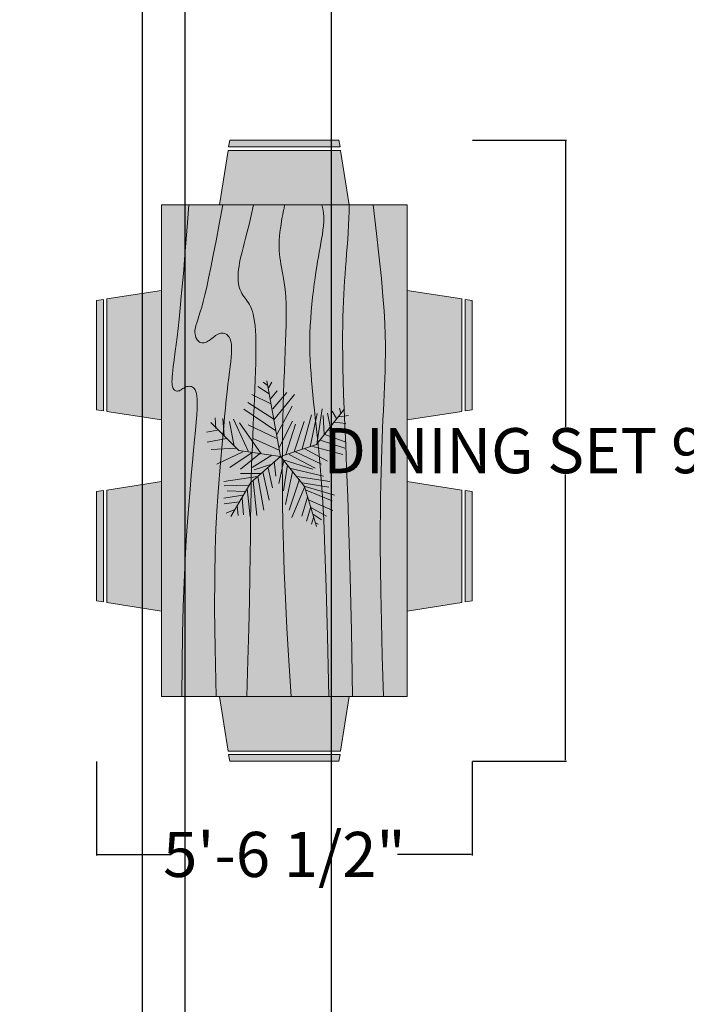
# Model space of a CAD drawing. Units: inches. Extents: x 853 to 1550, y 485 to 1596.
# Tile 9 of 18: x 1170 to 1288, y 1034 to 1208. Entities that reach past the tile are written whole.
import ezdxf

# ---------------------------------------------------------------- set-up
doc = ezdxf.new("R2010")
doc.units = ezdxf.units.IN
doc.header["$MEASUREMENT"] = 0
for name, color, linetype, lineweight in [('A-ANNO-DIMS', 2, 'Continuous', 18), ('furniture', 250, 'Continuous', 18), ('L-PLNT-TREE', 106, 'Continuous', 13)]:
    doc.layers.add(name, color=color, linetype=linetype, lineweight=lineweight)
doc.layers.add('A-FURN-PATT', color=254, linetype='Continuous', lineweight=13, true_color=0xfeeab9)
doc.styles.get("Standard").update_dxf_attribs({"font": 'arial.ttf'})
doc.dimstyles.get("Standard").update_dxf_attribs({"dimtxt": 8, "dimasz": 0.18, "dimexe": 0.18, "dimexo": 0.0625, "dimgap": 0.09, "dimtad": 0, "dimtih": 1, "dimtoh": 1, "dimzin": 0, "dimdsep": 46, "dimlunit": 3, "dimtxsty": 'Standard', "dimcen": 0.09, "dimadec": 0, "dimazin": 0, "dimtfac": 1, "dimtofl": 0, "dimtmove": 0, "dimatfit": 3, "dimfxl": 1, "dimtolj": 1, "dimtzin": 0, "dimarcsym": 0})

# ---------------------------------------------------------------- blocks, each defined once
blk = doc.blocks.new('Dining Set - 36 x 72 in.')
for p, q in [((-22, 27.5), (-22.1562, 26.50042)), ((-22, 27.5), (-6, 27.5)), ((-5.8437, 26.49966), (-6, 27.5)), ((6, 27.5), (5.8438, 26.50042)), ((6, 27.5), (22, 27.5)), ((22.1563, 26.49966), (22, 27.5)), ((-22.2343, 26.00059), (-23.4847, 17.99762)), ((-22.2304, 26), (-5.7608, 26)), ((-5.8416, 26.5), (-22.1534, 26.5)), ((-4.5152, 17.99762), (-5.7655, 25.99926)), ((5.7657, 26.00059), (4.5153, 17.99762)), ((5.7696, 26), (22.2392, 26)), ((22.1584, 26.5), (5.8466, 26.5)), ((23.4848, 17.99762), (22.2345, 25.99926)), ((36, 18), (-36, 18)), ((-36, 18), (-36, -18)), ((36, -18), (36, 18)), ((-44.0006, 8.23428), (-35.9976, 9.48474)), ((44.0006, 8.23428), (35.9976, 9.48474)), ((-45.5, 8), (-44.5004, 8.15617)), ((-45.5, 8), (-45.5, -8)), ((-44.5, -8.15843), (-44.5, 8.15338)), ((-44, 8.23041), (-44, -8.23915)), ((44, 8.23041), (44, -8.23915)), ((44.5, -8.15843), (44.5, 8.15338)), ((45.5, 8), (44.5005, 8.15617)), ((45.5, 8), (45.5, -8)), ((-44.4997, -8.15631), (-45.5, -8)), ((-35.9976, -9.48476), (-43.9993, -8.2345)), ((35.9976, -9.48476), (43.9993, -8.2345)), ((44.4997, -8.15631), (45.5, -8)), ((-36, -18), (36, -18)), ((-22.2343, -26.0006), (-23.4847, -17.99762)), ((-4.5152, -17.99762), (-5.7655, -25.99928)), ((5.7657, -26.0006), (4.5153, -17.99762)), ((23.4848, -17.99762), (22.2345, -25.99928)), ((-22.2304, -26), (-5.7608, -26)), ((-22, -27.5), (-22.1562, -26.50044)), ((-5.8416, -26.5), (-22.1534, -26.5)), ((-5.8437, -26.49967), (-6, -27.5)), ((5.7696, -26), (22.2392, -26)), ((6, -27.5), (5.8438, -26.50044)), ((22.1584, -26.5), (5.8466, -26.5)), ((22.1563, -26.49967), (22, -27.5)), ((-22, -27.5), (-6, -27.5)), ((6, -27.5), (22, -27.5))]:
    blk.add_line(p, q)
for points in [[(-36, 15), (-31.1772, 14.97754), (-26.8079, 14.91406), (-22.8538, 14.81543), (-19.276, 14.6875), (-16.0362, 14.53613), (-13.0957, 14.36718), (-10.4159, 14.18652), (-7.9583, 14), (-5.6904, 13.81315), (-3.6035, 13.63021), (-1.6954, 13.45508), (0.0365, 13.29166), (1.5945, 13.14388), (2.9811, 13.01562), (4.1988, 12.9108), (5.25, 12.83333), (6.1393, 12.78613), (6.8802, 12.76823), (7.4883, 12.77767), (7.9792, 12.8125), (8.3685, 12.87077), (8.6719, 12.95052), (8.9049, 13.0498), (9.0833, 13.16666), (9.2205, 13.29899), (9.3216, 13.44401), (9.3895, 13.59879), (9.4271, 13.76041), (9.4373, 13.92594), (9.4232, 14.09245), (9.3875, 14.257), (9.3333, 14.41666), (9.2638, 14.56917), (9.1836, 14.71484), (9.0975, 14.85465), (9.0104, 14.98958), (8.9272, 15.1206), (8.8529, 15.2487), (8.7922, 15.37483), (8.75, 15.5), (8.7305, 15.62467), (8.7344, 15.74739), (8.7617, 15.86621), (8.8125, 15.97916), (8.8867, 16.08431), (8.9844, 16.17968), (9.1055, 16.26334), (9.25, 16.33333), (9.4189, 16.38802), (9.6172, 16.42708), (9.8506, 16.45052), (10.125, 16.45833), (10.4463, 16.45052), (10.8203, 16.42708), (11.2529, 16.38802), (11.75, 16.33333), (12.3184, 16.26318), (12.9694, 16.17838), (13.7151, 16.07991), (14.5677, 15.96875), (15.5395, 15.84586), (16.6426, 15.71224), (17.8893, 15.56884), (19.2917, 15.41666), (20.859, 15.25667), (22.5879, 15.08984), (24.4721, 14.91715), (26.5052, 14.73958), (28.6809, 14.5581), (30.9929, 14.3737), (33.4347, 14.18733), (36, 14)], [(-36, 10), (-28.9766, 10.14274), (-23.1725, 10.20442), (-18.4241, 10.19775), (-14.5677, 10.13541), (-11.4399, 10.03011), (-8.877, 9.89453), (-6.7154, 9.74137), (-4.7917, 9.58333), (-2.9698, 9.43082), (-1.2246, 9.28515), (0.4415, 9.14534), (2.026, 9.01041), (3.5266, 8.87939), (4.9408, 8.7513), (6.266, 8.62516), (7.5, 8.5), (8.6411, 8.37549), (9.6914, 8.2539), (10.6538, 8.13818), (11.5312, 8.03125), (12.3267, 7.93603), (13.043, 7.85547), (13.6831, 7.79248), (14.25, 7.75), (14.7471, 7.7303), (15.1797, 7.73307), (15.5537, 7.75732), (15.875, 7.80208), (16.1494, 7.86637), (16.3828, 7.94922), (16.5811, 8.04964), (16.75, 8.16666), (16.8944, 8.29915), (17.0143, 8.44531), (17.1089, 8.60319), (17.1771, 8.77083), (17.218, 8.94629), (17.2305, 9.1276), (17.2137, 9.31282), (17.1667, 9.5), (17.0895, 9.6875), (16.987, 9.875), (16.8649, 10.0625), (16.7292, 10.25), (16.5856, 10.4375), (16.4401, 10.625), (16.2985, 10.8125), (16.1667, 11), (16.05, 11.18733), (15.9518, 11.3737), (15.8752, 11.5581), (15.8229, 11.73958), (15.798, 11.91715), (15.8034, 12.08984), (15.842, 12.25667), (15.9167, 12.41666), (16.0295, 12.56836), (16.1784, 12.70833), (16.3605, 12.83268), (16.5729, 12.9375), (16.8127, 13.01888), (17.0768, 13.07291), (17.3625, 13.0957), (17.6667, 13.08333), (17.9894, 13.03312), (18.3418, 12.94726), (18.7382, 12.82918), (19.1927, 12.68229), (19.7195, 12.51001), (20.3327, 12.31575), (21.0465, 12.10294), (21.875, 11.875), (22.8357, 11.63354), (23.959, 11.37304), (25.2786, 11.08618), (26.8282, 10.76562), (28.6414, 10.40405), (30.752, 9.99414), (33.1936, 9.52856), (36, 9)], [(-36, 5.5), (-30.7157, 5.3348), (-26.069, 5.20963), (-21.9946, 5.11767), (-18.4271, 5.05208), (-15.3009, 5.00602), (-12.5508, 4.97265), (-10.1112, 4.94515), (-7.9167, 4.91666), (-5.909, 4.88167), (-4.0586, 4.83984), (-2.3429, 4.79215), (-0.7396, 4.73958), (0.7739, 4.6831), (2.22, 4.6237), (3.6213, 4.56233), (5, 4.5), (6.373, 4.43782), (7.7344, 4.3776), (9.0723, 4.32129), (10.375, 4.27083), (11.6309, 4.22819), (12.8281, 4.19531), (13.9551, 4.17415), (15, 4.16666), (15.954, 4.17448), (16.819, 4.19791), (17.6001, 4.23698), (18.3021, 4.29166), (18.9299, 4.36198), (19.4883, 4.44791), (19.9823, 4.54948), (20.4167, 4.66666), (20.7969, 4.79899), (21.1302, 4.94401), (21.4245, 5.09879), (21.6875, 5.26041), (21.9271, 5.42594), (22.1511, 5.59245), (22.3672, 5.757), (22.5834, 5.91666), (22.8065, 6.06868), (23.0404, 6.21093), (23.2879, 6.34147), (23.5521, 6.45833), (23.8358, 6.55957), (24.142, 6.64323), (24.4735, 6.70735), (24.8334, 6.75), (25.2235, 6.76969), (25.642, 6.76692), (26.0858, 6.74267), (26.5521, 6.69791), (27.0379, 6.63362), (27.5404, 6.55078), (28.0565, 6.45036), (28.5834, 6.33333), (29.1242, 6.19987), (29.7071, 6.04687), (30.3661, 5.87044), (31.1354, 5.66666), (32.0493, 5.43164), (33.142, 5.16146), (34.4475, 4.85221), (36, 4.5)], [(-36, -1), (-30.7915, -0.6591), (-26.0195, -0.38216), (-21.6519, -0.16284), (-17.6563, 0.00521), (-14.0005, 0.12833), (-10.6523, 0.21289), (-7.5796, 0.26522), (-4.75, 0.29166), (-2.134, 0.29793), (0.2878, 0.28711), (2.5317, 0.26163), (4.6146, 0.22396), (6.5529, 0.17651), (8.3633, 0.12174), (10.0623, 0.06209), (11.6667, 0), (13.1899, -0.06201), (14.6341, -0.1211), (15.9982, -0.17432), (17.2813, -0.21875), (18.4823, -0.25147), (19.6003, -0.26953), (20.6343, -0.27002), (21.5834, -0.25), (22.4481, -0.20768), (23.2357, -0.14584), (23.9549, -0.06836), (24.6146, 0.02083), (25.2235, 0.11784), (25.7904, 0.21875), (26.3241, 0.31966), (26.8334, 0.41666), (27.3265, 0.50618), (27.8099, 0.58593), (28.2894, 0.65397), (28.7709, 0.70833), (29.2601, 0.74707), (29.763, 0.76823), (30.2855, 0.76985), (30.8334, 0.75), (31.4088, 0.70784), (31.9994, 0.64713), (32.589, 0.57275), (33.1615, 0.48958), (33.7008, 0.4025), (34.1908, 0.3164), (34.6153, 0.23616), (34.9584, 0.16666), (35.2099, 0.11165), (35.3848, 0.07031), (35.504, 0.04069), (35.5886, 0.02083), (35.6594, 0.00879), (35.7377, 0.0026), (35.8442, 0.00032), (36, 0)], [(-36, -6.5), (-27.1843, -6.31267), (-20.084, -6.1263), (-14.469, -5.9419), (-10.1094, -5.76042), (-6.7752, -5.58285), (-4.2363, -5.41016), (-2.2629, -5.24333), (-0.625, -5.08334), (0.8708, -4.93099), (2.2715, -4.78646), (3.5872, -4.64974), (4.8281, -4.52084), (6.0046, -4.39974), (7.127, -4.28646), (8.2053, -4.18099), (9.25, -4.08334), (10.2705, -3.99382), (11.2734, -3.91407), (12.2647, -3.84603), (13.25, -3.79167), (14.2354, -3.75293), (15.2266, -3.73177), (16.2295, -3.73015), (17.25, -3.75), (18.2912, -3.79248), (19.3451, -3.85547), (20.4009, -3.93604), (21.4479, -4.03125), (22.4754, -4.13819), (23.4727, -4.25391), (24.4289, -4.37549), (25.3334, -4.5), (26.1785, -4.62492), (26.9694, -4.74935), (27.7145, -4.87281), (28.4219, -4.99479), (29.1, -5.11483), (29.7572, -5.23242), (30.4016, -5.34709), (31.0417, -5.45834), (31.6837, -5.56437), (32.3262, -5.65821), (32.9658, -5.73153), (33.599, -5.77604), (34.2224, -5.78345), (34.8327, -5.74545), (35.4264, -5.65373), (36, -5.5)], [(-36, -10), (-26.4022, -9.81299), (-18.4675, -9.62891), (-11.9839, -9.45069), (-6.7396, -9.28125), (-2.5226, -9.12354), (0.8789, -8.98047), (3.6769, -8.85498), (6.0833, -8.75), (8.2767, -8.66765), (10.3021, -8.60677), (12.1712, -8.56543), (13.8958, -8.54167), (15.4876, -8.53353), (16.9583, -8.53907), (18.3197, -8.55632), (19.5834, -8.58334), (20.7616, -8.61841), (21.8685, -8.66081), (22.9188, -8.71004), (23.9271, -8.76563), (24.9081, -8.82707), (25.8763, -8.89388), (26.8465, -8.96558), (27.8334, -9.04167), (28.8474, -9.12118), (29.8828, -9.20117), (30.93, -9.27824), (31.9792, -9.34896), (33.0205, -9.40991), (34.0443, -9.45768), (35.0407, -9.48885), (36, -9.5)], [(-36, -14.5), (-30.0881, -14.33513), (-25.0332, -14.21224), (-20.7312, -14.12647), (-17.0781, -14.07292), (-13.97, -14.04671), (-11.3027, -14.04297), (-8.9724, -14.05681), (-6.875, -14.08334), (-4.9224, -14.11833), (-3.0905, -14.16016), (-1.3709, -14.20785), (0.2448, -14.26042), (1.7647, -14.3169), (3.1973, -14.3763), (4.5507, -14.43767), (5.8333, -14.5), (7.0554, -14.5621), (8.235, -14.62175), (9.3922, -14.67652), (10.5469, -14.72396), (11.7192, -14.76164), (12.929, -14.78711), (14.1965, -14.79794), (15.5417, -14.79167), (16.9933, -14.76424), (18.6152, -14.70508), (20.4804, -14.60197), (22.6615, -14.44271), (25.2312, -14.21509), (28.2624, -13.9069), (31.8277, -13.50594), (36, -13)]]:
    blk.add_lwpolyline(points)
blk = doc.blocks.new('dining area')
at = {"layer": 'furniture', "xscale": 0.6659924291999282, "yscale": 0.6659924291999282, "zscale": 0.6659924291999282, "rotation": 90}
blk.add_blockref('Dining Set - 36 x 72 in.', (-0.439, 20.507), dxfattribs=at)
blk = doc.blocks.new('*U18')
for p, q in [((-8.737, 47.138), (-17.069, 52.711)), ((-10.186, 53.64), (-13.084, 55.962)), ((0, 0), (-10.5, 57)), ((-9.099, 51.782), (-6.563, 55.962)), ((-7.288, 39.707), (-21.778, 46.673)), ((-7.65, 43.423), (-2.578, 49.46)), ((-5.839, 35.992), (4.667, 48.067)), ((-5.114, 27.632), (10.463, 46.673)), ((-5.114, 28.097), (-24.676, 40.636)), ((-2.941, 16.486), (8.652, 37.85)), ((-3.665, 19.273), (-27.574, 35.527)), ((16.259, 5.805), (23.142, 31.348)), ((22.055, 7.198), (27.489, 32.277)), ((27, 9), (48, 36)), ((27.127, 9.056), (31.112, 35.992)), ((31.836, 30.883), (32.561, 16.486)), ((35.096, 32.741), (37.27, 22.524)), ((38.719, 34.134), (41.979, 28.561)), ((43.791, 29.954), (51.036, 30.883)), ((44.153, 36.456), (45.239, 32.741)), ((-31.5, 4.5), (-52.5, 25.5)), ((-48.585, 21.131), (-49.309, 29.026)), ((-43.513, 28.561), (-42.427, 15.558)), ((-38.442, 26.239), (-34.819, 7.663)), ((-35.544, 28.097), (-24.314, 3.947)), ((-14.533, 2.09), (-30.834, 25.31)), ((-24.314, 23.917), (-2.941, 13.7)), ((-1.129, 6.734), (9.014, 26.704)), ((3.942, 1.625), (11.187, 24.381)), ((10.101, 3.483), (17.708, 26.239)), ((40.53, 25.775), (48.862, 24.846)), ((-47.498, 19.737), (-55.83, 18.344)), ((33.285, 16.486), (48.862, 10.913)), ((36.183, 19.737), (48.137, 17.88)), ((-40.615, 13.7), (-55.105, 10.913)), ((-20.691, 13.7), (-1.129, 4.876)), ((0, 0), (27, 9)), ((24.229, 7.663), (46.688, 1.625)), ((29.662, 12.307), (48.137, 6.269)), ((-33.37, 6.269), (-52.207, 5.34)), ((-28.299, 3.483), (-47.86, -5.805)), ((-21.416, 3.018), (-38.079, -8.128)), ((0, 0), (-31.5, 4.5)), ((-15.982, 2.09), (-30.11, -9.521)), ((0, 0), (-22.5, -19.5)), ((-6.563, 1.161), (-21.416, -8.128)), ((0, 0), (18, -22.5)), ((6.478, 1.625), (26.04, -8.592)), ((11.187, 3.483), (30.749, -5.805)), ((18.07, 5.805), (35.096, -3.483)), ((-6.563, -5.805), (-19.967, -9.985)), ((-4.752, -3.483), (-3.665, -14.629)), ((2.493, -3.019), (-1.491, -20.202)), ((1.769, -2.555), (24.229, -9.521)), ((5.029, -6.27), (2.131, -25.775)), ((-15.257, -12.772), (-30.11, -12.772)), ((-13.446, -11.378), (-8.737, -32.741)), ((-9.461, -8.592), (-6.201, -23.453)), ((9.014, -11.378), (3.58, -35.992)), ((7.565, -9.056), (32.198, -14.629)), ((-17.431, -15.094), (-42.789, -18.809)), ((-24.314, -21.596), (-42.427, -22.06)), ((-22.5, -19.5), (-37.5, -45)), ((-20.691, -18.345), (-17.793, -44.352)), ((-17.069, -15.094), (-12.721, -40.172)), ((14.085, -16.951), (6.478, -40.172)), ((12.274, -15.094), (36.907, -18.809)), ((16.259, -19.738), (36.183, -22.989)), ((-28.299, -29.026), (-42.789, -31.348)), ((-26.849, -26.24), (-40.253, -25.775)), ((-25.038, -23.918), (-22.865, -45.281)), ((18.07, -22.524), (8.289, -45.745)), ((18, -22.5), (27, -52.5)), ((18.433, -22.524), (40.53, -29.026)), ((19.157, -25.311), (38.719, -33.206)), ((-30.834, -34.135), (-42.427, -35.528)), ((-32.646, -36.921), (-31.921, -44.352)), ((-29.023, -30.884), (-27.936, -43.887)), ((20.244, -30.419), (15.897, -44.816)), ((21.331, -32.741), (39.081, -40.636)), ((-34.457, -39.708), (-40.978, -42.494)), ((22.78, -37.85), (19.519, -48.532)), ((22.78, -38.314), (34.372, -44.816)), ((24.591, -43.423), (30.749, -47.603)), ((24.591, -45.745), (23.142, -50.854)), ((26.764, -49.925), (28.213, -50.854))]:
    blk.add_line(p, q)
blk = doc.blocks.new('*D67')
at = {"layer": 'A-ANNO-DIMS', "color": 0, "lineweight": -2, "transparency": 16777216}
for p, q in [((1250.4, 1186.71), (1267.03, 1186.71)), ((1266.85, 1186.53), (1266.85, 1135.89)), ((1266.85, 1076.81), (1266.85, 1127.44)), ((1250.4, 1076.63), (1267.03, 1076.63))]:
    blk.add_line(p, q, dxfattribs=at)
at = {"layer": 'A-ANNO-DIMS', "color": 0, "transparency": 16777216}
for points in [[(1266.82, 1186.53), (1266.88, 1186.53), (1266.85, 1186.71)], [(1266.82, 1076.81), (1266.88, 1076.81), (1266.85, 1076.63)]]:
    blk.add_solid(points, dxfattribs=at)
at = {"layer": 'Defpoints', "color": 0, "transparency": 16777216}
for p in [(1250.34, 1186.71), (1266.85, 1186.71), (1250.34, 1076.63)]:
    blk.add_point(p, dxfattribs=at)
at = {"layer": 'A-ANNO-DIMS', "color": 0, "transparency": 16777216, "insert": (1266.85, 1131.67), "char_height": 8, "attachment_point": 5}
blk.add_mtext('\\A1;DINING SET 9\'-2"', dxfattribs=at)
blk = doc.blocks.new('*D68')
at = {"layer": 'A-ANNO-DIMS', "color": 0, "lineweight": -2, "transparency": 16777216}
for p, q in [((1183.81, 1076.57), (1183.81, 1059.94)), ((1250.34, 1076.57), (1250.34, 1059.94)), ((1183.99, 1060.12), (1197.03, 1060.12)), ((1250.16, 1060.12), (1237.12, 1060.12))]:
    blk.add_line(p, q, dxfattribs=at)
at = {"layer": 'A-ANNO-DIMS', "color": 0, "transparency": 16777216}
for points in [[(1183.99, 1060.15), (1183.99, 1060.09), (1183.81, 1060.12)], [(1250.16, 1060.15), (1250.16, 1060.09), (1250.34, 1060.12)]]:
    blk.add_solid(points, dxfattribs=at)
at = {"layer": 'Defpoints', "color": 0, "transparency": 16777216}
for p in [(1183.81, 1076.63), (1250.34, 1076.63), (1250.34, 1060.12)]:
    blk.add_point(p, dxfattribs=at)
at = {"layer": 'A-ANNO-DIMS', "color": 0, "transparency": 16777216, "insert": (1217.08, 1060.12), "char_height": 8, "attachment_point": 5}
blk.add_mtext('\\A1;5\'-6 1/2"', dxfattribs=at)
blk = doc.blocks.new('*D72')
at = {"layer": 'A-ANNO-DIMS', "color": 0, "lineweight": -2, "transparency": 16777216}
for p, q in [((1139.44, 1321.07), (1139.44, 497.1)), ((1199.44, 1321.07), (1199.44, 497.1)), ((1139.62, 497.28), (1158.71, 497.28)), ((1199.26, 497.28), (1180.16, 497.28))]:
    blk.add_line(p, q, dxfattribs=at)
at = {"layer": 'A-ANNO-DIMS', "color": 0, "transparency": 16777216}
for points in [[(1139.62, 497.31), (1139.62, 497.25), (1139.44, 497.28)], [(1199.26, 497.31), (1199.26, 497.25), (1199.44, 497.28)]]:
    blk.add_solid(points, dxfattribs=at)
at = {"layer": 'Defpoints', "color": 0, "transparency": 16777216}
for p in [(1139.44, 1321.13), (1199.44, 1321.13), (1199.44, 497.28)]:
    blk.add_point(p, dxfattribs=at)
at = {"layer": 'A-ANNO-DIMS', "color": 0, "transparency": 16777216, "insert": (1169.44, 497.28), "char_height": 8, "attachment_point": 5}
blk.add_mtext('\\A1;5\'-0"', dxfattribs=at)
blk = doc.blocks.new('*D81')
at = {"layer": 'A-ANNO-DIMS', "color": 0, "lineweight": -2, "transparency": 16777216}
for p, q in [((1191.94, 767.69), (1191.94, 1584.65)), ((1192.12, 1584.47), (1225.27, 1584.47)), ((1225.45, 767.69), (1225.45, 1584.65)), ((1225.45, 1584.47), (1225.63, 1584.47))]:
    blk.add_line(p, q, dxfattribs=at)
at = {"layer": 'A-ANNO-DIMS', "color": 0, "transparency": 16777216}
for points in [[(1192.12, 1584.5), (1192.12, 1584.44), (1191.94, 1584.47)], [(1225.27, 1584.5), (1225.27, 1584.44), (1225.45, 1584.47)]]:
    blk.add_solid(points, dxfattribs=at)
at = {"layer": 'Defpoints', "color": 0, "transparency": 16777216}
for p in [(1225.45, 1584.47), (1191.94, 767.63), (1225.45, 767.63)]:
    blk.add_point(p, dxfattribs=at)
at = {"layer": 'A-ANNO-DIMS', "color": 0, "transparency": 16777216, "insert": (1245.74, 1584.47), "char_height": 8, "attachment_point": 5}
blk.add_mtext('\\A1;2\'-9 1/2"', dxfattribs=at)

msp = doc.modelspace()

# ---------------------------------------------------------------- hatches: boundary and pattern name
at = {"layer": 'A-FURN-PATT'}
h = msp.add_hatch(color=256, dxfattribs=at)
h.dxf.hatch_style = 1
h.paths.add_polyline_path([(1195.302, 1126.206), (1185.625, 1124.693), (1185.625, 1104.772), (1195.302, 1103.26)])
h.paths.add_polyline_path([(1195.302, 1160.075), (1185.625, 1158.563), (1185.625, 1138.642), (1195.302, 1137.13)])
h.paths.add_polyline_path([(1248.526, 1158.563), (1238.849, 1160.075), (1238.849, 1137.13), (1248.526, 1138.642)])
h.paths.add_polyline_path([(1248.526, 1124.693), (1238.849, 1126.206), (1238.849, 1103.26), (1248.526, 1104.772)])
h.paths.add_polyline_path([(1228.548, 1088.121), (1205.602, 1088.121), (1207.114, 1078.444), (1227.036, 1078.444)])
h.paths.add_polyline_path([(1227.036, 1184.892), (1207.114, 1184.892), (1205.602, 1175.215), (1228.548, 1175.215)])
h.paths.add_polyline_path([(1226.752, 1186.706), (1207.398, 1186.706), (1207.209, 1185.496), (1226.941, 1185.496)])
h.paths.add_polyline_path([(1185.02, 1158.469), (1183.81, 1158.28), (1183.81, 1138.926), (1185.02, 1138.736)])
h.paths.add_polyline_path([(1185.02, 1124.599), (1183.81, 1124.41), (1183.81, 1105.056), (1185.02, 1104.867)])
h.paths.add_polyline_path([(1226.941, 1077.839), (1207.209, 1077.839), (1207.398, 1076.629), (1226.752, 1076.629)])
h.paths.add_polyline_path([(1250.34, 1124.41), (1249.13, 1124.599), (1249.13, 1104.867), (1250.34, 1105.056)])
h.paths.add_polyline_path([(1250.34, 1158.28), (1249.13, 1158.469), (1249.13, 1138.736), (1250.34, 1138.926)])
h = msp.add_hatch(color=256, dxfattribs=at)
h.dxf.hatch_style = 1
h.paths.add_polyline_path([(1200.997, 1131.712), (1201.176, 1133.596), (1201.331, 1135.274), (1201.458, 1136.747), (1201.551, 1138.018), (1201.609, 1139.094), (1201.63, 1139.99), (1201.619, 1140.726), (1201.577, 1141.32), (1201.506, 1141.791), (1201.41, 1142.158), (1201.29, 1142.439), (1201.148, 1142.655), (1200.988, 1142.821), (1200.813, 1142.943), (1200.626, 1143.026), (1200.43, 1143.071), (1200.23, 1143.083), (1200.028, 1143.066), (1199.829, 1143.023), (1199.636, 1142.958), (1199.452, 1142.874), (1199.275, 1142.777), (1199.106, 1142.672), (1198.81, 1142.481), (1198.539, 1142.324), (1198.249, 1142.226), (1197.951, 1142.236), (1197.676, 1142.359), (1197.444, 1142.597), (1197.318, 1142.857), (1197.252, 1143.061), (1197.204, 1143.301), (1197.176, 1143.583), (1197.167, 1143.915), (1197.176, 1144.304), (1197.204, 1144.756), (1197.252, 1145.28), (1197.318, 1145.881), (1197.403, 1146.568), (1197.505, 1147.356), (1197.624, 1148.258), (1197.759, 1149.289), (1197.907, 1150.465), (1198.069, 1151.799), (1198.242, 1153.307), (1198.427, 1155.004), (1198.62, 1156.899), (1198.822, 1158.991), (1199.031, 1161.27), (1199.246, 1163.729), (1199.465, 1166.361), (1199.688, 1169.158), (1199.914, 1172.111), (1200.14, 1175.215), (1195.302, 1175.215), (1195.302, 1088.121), (1198.931, 1088.121), (1198.958, 1093.955), (1199.035, 1099.24), (1199.154, 1104.023), (1199.309, 1108.351), (1199.492, 1112.27), (1199.696, 1115.827), (1199.915, 1119.068), (1200.14, 1122.041), (1200.366, 1124.784), (1200.588, 1127.309), (1200.799, 1129.617)])
h.paths.add_polyline_path([(1207.091, 1143.391), (1207.231, 1144.555), (1207.36, 1145.616), (1207.475, 1146.579), (1207.573, 1147.445), (1207.649, 1148.219), (1207.7, 1148.905), (1207.724, 1149.506), (1207.721, 1150.03), (1207.692, 1150.482), (1207.637, 1150.871), (1207.56, 1151.203), (1207.459, 1151.485), (1207.338, 1151.725), (1207.196, 1151.929), (1207.036, 1152.104), (1206.859, 1152.249), (1206.668, 1152.363), (1206.466, 1152.446), (1206.253, 1152.495), (1206.034, 1152.51), (1205.81, 1152.49), (1205.584, 1152.433), (1205.357, 1152.34), (1205.13, 1152.216), (1204.903, 1152.068), (1204.676, 1151.904), (1204.45, 1151.73), (1204.223, 1151.554), (1203.996, 1151.383), (1203.769, 1151.224), (1203.542, 1151.082), (1203.317, 1150.964), (1203.094, 1150.871), (1202.874, 1150.808), (1202.547, 1150.762), (1202.249, 1150.831), (1202.055, 1150.921), (1201.872, 1151.058), (1201.703, 1151.238), (1201.552, 1151.458), (1201.425, 1151.715), (1201.327, 1152.005), (1201.262, 1152.324), (1201.234, 1152.67), (1201.249, 1153.038), (1201.31, 1153.428), (1201.414, 1153.855), (1201.556, 1154.334), (1201.734, 1154.884), (1201.943, 1155.521), (1202.178, 1156.263), (1202.435, 1157.126), (1202.711, 1158.128), (1203.003, 1159.291), (1203.318, 1160.649), (1203.665, 1162.246), (1204.053, 1164.12), (1204.49, 1166.313), (1204.986, 1168.866), (1205.549, 1171.82), (1206.188, 1175.215), (1200.14, 1175.215), (1199.914, 1172.111), (1199.688, 1169.158), (1199.465, 1166.361), (1199.246, 1163.729), (1199.031, 1161.27), (1198.822, 1158.991), (1198.62, 1156.899), (1198.427, 1155.004), (1198.242, 1153.307), (1198.069, 1151.799), (1197.907, 1150.465), (1197.759, 1149.289), (1197.624, 1148.258), (1197.505, 1147.356), (1197.403, 1146.568), (1197.318, 1145.881), (1197.252, 1145.28), (1197.204, 1144.756), (1197.176, 1144.304), (1197.167, 1143.915), (1197.176, 1143.583), (1197.204, 1143.301), (1197.252, 1143.061), (1197.318, 1142.857), (1197.402, 1142.682), (1197.504, 1142.536), (1197.619, 1142.417), (1197.746, 1142.328), (1197.883, 1142.266), (1198.026, 1142.233), (1198.175, 1142.228), (1198.326, 1142.252), (1198.477, 1142.303), (1198.63, 1142.376), (1198.785, 1142.466), (1198.943, 1142.567), (1199.223, 1142.747), (1199.553, 1142.929), (1199.933, 1143.058), (1200.338, 1143.093), (1200.626, 1143.026), (1200.813, 1142.943), (1200.988, 1142.821), (1201.148, 1142.655), (1201.29, 1142.439), (1201.41, 1142.158), (1201.506, 1141.791), (1201.577, 1141.32), (1201.619, 1140.726), (1201.63, 1139.99), (1201.609, 1139.094), (1201.551, 1138.018), (1201.458, 1136.747), (1201.331, 1135.274), (1201.176, 1133.596), (1200.997, 1131.712), (1200.799, 1129.617), (1200.588, 1127.309), (1200.366, 1124.784), (1200.14, 1122.041), (1199.915, 1119.068), (1199.696, 1115.827), (1199.492, 1112.27), (1199.309, 1108.351), (1199.154, 1104.023), (1199.035, 1099.24), (1198.958, 1093.955), (1198.931, 1088.121), (1204.979, 1088.121), (1204.806, 1096.617), (1204.731, 1103.637), (1204.74, 1109.381), (1204.815, 1114.046), (1204.942, 1117.83), (1205.106, 1120.93), (1205.292, 1123.545), (1205.483, 1125.872), (1205.667, 1128.075), (1205.843, 1130.186), (1206.013, 1132.202), (1206.176, 1134.118), (1206.334, 1135.934), (1206.489, 1137.644), (1206.642, 1139.247), (1206.793, 1140.74), (1206.944, 1142.12)])
h.paths.add_polyline_path([(1211.961, 1145.737), (1212, 1147.185), (1212.026, 1148.548), (1212.035, 1149.812), (1212.025, 1150.966), (1211.997, 1152.013), (1211.95, 1152.957), (1211.884, 1153.807), (1211.799, 1154.566), (1211.695, 1155.241), (1211.572, 1155.839), (1211.43, 1156.364), (1211.27, 1156.824), (1211.095, 1157.228), (1210.907, 1157.584), (1210.712, 1157.902), (1210.512, 1158.192), (1210.31, 1158.462), (1210.111, 1158.724), (1209.918, 1158.985), (1209.734, 1159.255), (1209.562, 1159.538), (1209.404, 1159.838), (1209.263, 1160.157), (1209.14, 1160.5), (1209.039, 1160.871), (1208.962, 1161.272), (1208.91, 1161.707), (1208.886, 1162.179), (1208.89, 1162.685), (1208.919, 1163.222), (1208.973, 1163.786), (1209.051, 1164.374), (1209.151, 1164.982), (1209.273, 1165.606), (1209.414, 1166.243), (1209.576, 1166.897), (1209.761, 1167.602), (1209.974, 1168.4), (1210.22, 1169.33), (1210.505, 1170.436), (1210.832, 1171.757), (1211.206, 1173.337), (1211.632, 1175.215), (1206.188, 1175.215), (1205.549, 1171.82), (1204.986, 1168.866), (1204.49, 1166.313), (1204.053, 1164.12), (1203.665, 1162.246), (1203.318, 1160.649), (1203.003, 1159.291), (1202.711, 1158.128), (1202.435, 1157.126), (1202.178, 1156.263), (1201.943, 1155.521), (1201.734, 1154.884), (1201.556, 1154.334), (1201.414, 1153.855), (1201.31, 1153.428), (1201.249, 1153.038), (1201.234, 1152.67), (1201.262, 1152.324), (1201.327, 1152.005), (1201.425, 1151.715), (1201.552, 1151.458), (1201.703, 1151.238), (1201.872, 1151.058), (1202.055, 1150.921), (1202.249, 1150.831), (1202.451, 1150.784), (1202.66, 1150.778), (1202.874, 1150.808), (1203.094, 1150.871), (1203.317, 1150.964), (1203.542, 1151.082), (1203.769, 1151.224), (1203.996, 1151.383), (1204.223, 1151.554), (1204.45, 1151.73), (1204.82, 1152.014), (1205.13, 1152.216), (1205.357, 1152.34), (1205.584, 1152.433), (1205.81, 1152.49), (1206.034, 1152.51), (1206.253, 1152.495), (1206.466, 1152.446), (1206.668, 1152.363), (1206.859, 1152.249), (1207.036, 1152.104), (1207.196, 1151.929), (1207.338, 1151.725), (1207.459, 1151.485), (1207.56, 1151.203), (1207.637, 1150.871), (1207.692, 1150.482), (1207.721, 1150.03), (1207.724, 1149.506), (1207.7, 1148.905), (1207.649, 1148.219), (1207.573, 1147.445), (1207.475, 1146.579), (1207.36, 1145.616), (1207.231, 1144.555), (1207.091, 1143.391), (1206.944, 1142.12), (1206.793, 1140.74), (1206.642, 1139.247), (1206.489, 1137.644), (1206.334, 1135.934), (1206.176, 1134.118), (1206.013, 1132.202), (1205.843, 1130.186), (1205.667, 1128.075), (1205.483, 1125.872), (1205.292, 1123.545), (1205.106, 1120.93), (1204.942, 1117.83), (1204.815, 1114.046), (1204.74, 1109.381), (1204.731, 1103.637), (1204.806, 1096.617), (1204.979, 1088.121), (1210.422, 1088.121), (1210.622, 1094.513), (1210.773, 1100.134), (1210.885, 1105.062), (1210.964, 1109.378), (1211.02, 1113.159), (1211.06, 1116.486), (1211.093, 1119.437), (1211.128, 1122.091), (1211.17, 1124.52), (1211.221, 1126.758), (1211.278, 1128.834), (1211.342, 1130.773), (1211.41, 1132.604), (1211.482, 1134.353), (1211.556, 1136.048), (1211.632, 1137.716), (1211.707, 1139.377), (1211.78, 1141.024), (1211.848, 1142.642), (1211.909, 1144.218)])
h.paths.add_polyline_path([(1216.928, 1141.784), (1217, 1143.839), (1217.075, 1145.78), (1217.15, 1147.623), (1217.222, 1149.37), (1217.286, 1151.02), (1217.34, 1152.572), (1217.379, 1154.025), (1217.401, 1155.377), (1217.402, 1156.628), (1217.377, 1157.776), (1217.326, 1158.822), (1217.251, 1159.774), (1217.158, 1160.644), (1217.05, 1161.442), (1216.933, 1162.179), (1216.81, 1162.865), (1216.688, 1163.51), (1216.571, 1164.126), (1216.463, 1164.723), (1216.366, 1165.308), (1216.284, 1165.888), (1216.218, 1166.47), (1216.171, 1167.062), (1216.146, 1167.67), (1216.144, 1168.302), (1216.168, 1168.965), (1216.219, 1169.661), (1216.292, 1170.375), (1216.382, 1171.089), (1216.483, 1171.781), (1216.588, 1172.433), (1216.692, 1173.026), (1216.789, 1173.54), (1216.873, 1173.955), (1216.94, 1174.259), (1216.99, 1174.47), (1217.026, 1174.615), (1217.05, 1174.717), (1217.064, 1174.803), (1217.072, 1174.897), (1217.075, 1175.026), (1217.075, 1175.215), (1211.632, 1175.215), (1211.206, 1173.337), (1210.832, 1171.757), (1210.505, 1170.436), (1210.22, 1169.33), (1209.974, 1168.4), (1209.761, 1167.602), (1209.576, 1166.897), (1209.414, 1166.243), (1209.273, 1165.606), (1209.151, 1164.982), (1209.051, 1164.374), (1208.973, 1163.786), (1208.919, 1163.222), (1208.89, 1162.685), (1208.886, 1162.179), (1208.91, 1161.707), (1208.962, 1161.272), (1209.039, 1160.871), (1209.14, 1160.5), (1209.263, 1160.157), (1209.404, 1159.838), (1209.562, 1159.538), (1209.734, 1159.255), (1209.918, 1158.985), (1210.111, 1158.724), (1210.31, 1158.462), (1210.512, 1158.192), (1210.712, 1157.902), (1210.907, 1157.584), (1211.095, 1157.228), (1211.27, 1156.824), (1211.43, 1156.364), (1211.572, 1155.839), (1211.695, 1155.241), (1211.799, 1154.566), (1211.884, 1153.807), (1211.95, 1152.957), (1211.997, 1152.013), (1212.025, 1150.966), (1212.035, 1149.812), (1212.026, 1148.548), (1212, 1147.185), (1211.961, 1145.737), (1211.909, 1144.218), (1211.848, 1142.642), (1211.78, 1141.024), (1211.707, 1139.377), (1211.632, 1137.716), (1211.556, 1136.048), (1211.482, 1134.353), (1211.41, 1132.604), (1211.342, 1130.773), (1211.278, 1128.834), (1211.221, 1126.758), (1211.17, 1124.52), (1211.128, 1122.091), (1211.093, 1119.437), (1211.06, 1116.486), (1211.02, 1113.159), (1210.964, 1109.378), (1210.885, 1105.062), (1210.773, 1100.134), (1210.622, 1094.513), (1210.422, 1088.121), (1218.285, 1088.121), (1217.872, 1094.421), (1217.537, 1100.194), (1217.272, 1105.477), (1217.069, 1110.31), (1216.92, 1114.732), (1216.818, 1118.782), (1216.754, 1122.499), (1216.722, 1125.922), (1216.715, 1129.086), (1216.728, 1132.016), (1216.759, 1134.73), (1216.804, 1137.25), (1216.862, 1139.594)])
h.paths.add_polyline_path([(1222.865, 1134.415), (1222.7, 1136.007), (1222.544, 1137.508), (1222.397, 1138.931), (1222.26, 1140.289), (1222.133, 1141.593), (1222.014, 1142.857), (1221.906, 1144.091), (1221.81, 1145.304), (1221.727, 1146.504), (1221.662, 1147.695), (1221.615, 1148.887), (1221.589, 1150.086), (1221.587, 1151.299), (1221.611, 1152.534), (1221.663, 1153.793), (1221.739, 1155.068), (1221.836, 1156.345), (1221.951, 1157.612), (1222.081, 1158.855), (1222.221, 1160.061), (1222.368, 1161.218), (1222.518, 1162.312), (1222.67, 1163.334), (1222.82, 1164.291), (1222.969, 1165.192), (1223.117, 1166.048), (1223.262, 1166.868), (1223.404, 1167.663), (1223.543, 1168.443), (1223.678, 1169.217), (1223.806, 1169.993), (1223.919, 1170.771), (1224.008, 1171.544), (1224.062, 1172.31), (1224.071, 1173.064), (1224.025, 1173.803), (1223.914, 1174.521), (1223.728, 1175.215), (1217.075, 1175.215), (1217.074, 1174.861), (1217.047, 1174.699), (1216.99, 1174.47), (1216.94, 1174.259), (1216.873, 1173.955), (1216.789, 1173.54), (1216.692, 1173.026), (1216.588, 1172.433), (1216.483, 1171.781), (1216.382, 1171.089), (1216.292, 1170.375), (1216.219, 1169.661), (1216.168, 1168.965), (1216.144, 1168.302), (1216.146, 1167.67), (1216.171, 1167.062), (1216.218, 1166.47), (1216.284, 1165.888), (1216.366, 1165.308), (1216.463, 1164.723), (1216.571, 1164.126), (1216.688, 1163.51), (1216.81, 1162.865), (1216.933, 1162.179), (1217.05, 1161.442), (1217.158, 1160.644), (1217.251, 1159.774), (1217.326, 1158.822), (1217.377, 1157.776), (1217.402, 1156.628), (1217.401, 1155.377), (1217.379, 1154.025), (1217.34, 1152.572), (1217.286, 1151.02), (1217.222, 1149.37), (1217.15, 1147.623), (1217.075, 1145.78), (1217, 1143.839), (1216.928, 1141.784), (1216.862, 1139.594), (1216.804, 1137.25), (1216.759, 1134.73), (1216.728, 1132.016), (1216.715, 1129.086), (1216.722, 1125.922), (1216.754, 1122.499), (1216.818, 1118.782), (1216.92, 1114.732), (1217.069, 1110.31), (1217.272, 1105.477), (1217.537, 1100.194), (1217.872, 1094.421), (1218.285, 1088.121), (1224.938, 1088.121), (1224.711, 1098.785), (1224.486, 1107.373), (1224.263, 1114.166), (1224.043, 1119.439), (1223.828, 1123.472), (1223.619, 1126.543), (1223.418, 1128.93), (1223.224, 1130.912), (1223.04, 1132.721)])
h.paths.add_polyline_path([(1234.886, 1144.426), (1234.931, 1145.844), (1234.962, 1147.307), (1234.975, 1148.84), (1234.968, 1150.467), (1234.934, 1152.223), (1234.863, 1154.185), (1234.738, 1156.442), (1234.545, 1159.08), (1234.27, 1162.188), (1233.897, 1165.855), (1233.412, 1170.168), (1232.8, 1175.215), (1223.728, 1175.215), (1223.914, 1174.521), (1224.025, 1173.803), (1224.071, 1173.064), (1224.062, 1172.31), (1224.008, 1171.544), (1223.919, 1170.771), (1223.806, 1169.993), (1223.678, 1169.217), (1223.543, 1168.443), (1223.404, 1167.663), (1223.262, 1166.868), (1223.117, 1166.048), (1222.969, 1165.192), (1222.82, 1164.291), (1222.67, 1163.334), (1222.518, 1162.312), (1222.368, 1161.218), (1222.221, 1160.061), (1222.081, 1158.855), (1221.951, 1157.612), (1221.836, 1156.345), (1221.739, 1155.068), (1221.663, 1153.793), (1221.611, 1152.534), (1221.587, 1151.299), (1221.589, 1150.086), (1221.615, 1148.887), (1221.662, 1147.695), (1221.727, 1146.504), (1221.81, 1145.304), (1221.906, 1144.091), (1222.014, 1142.857), (1222.133, 1141.593), (1222.26, 1140.289), (1222.397, 1138.931), (1222.544, 1137.508), (1222.7, 1136.007), (1222.865, 1134.415), (1223.04, 1132.721), (1223.224, 1130.912), (1223.418, 1128.93), (1223.619, 1126.543), (1223.828, 1123.472), (1224.043, 1119.439), (1224.263, 1114.166), (1224.486, 1107.373), (1224.711, 1098.785), (1224.938, 1088.121), (1234.615, 1088.121), (1234.415, 1095.272), (1234.267, 1101.387), (1234.163, 1106.591), (1234.098, 1111.009), (1234.066, 1114.769), (1234.062, 1117.996), (1234.079, 1120.814), (1234.111, 1123.351), (1234.153, 1125.713), (1234.204, 1127.929), (1234.261, 1130.009), (1234.325, 1131.964), (1234.393, 1133.802), (1234.465, 1135.535), (1234.539, 1137.172), (1234.615, 1138.724), (1234.69, 1140.202), (1234.762, 1141.629), (1234.828, 1143.029)])
h.paths.add_polyline_path([(1238.849, 1175.215), (1232.8, 1175.215), (1233.412, 1170.168), (1233.897, 1165.855), (1234.27, 1162.188), (1234.545, 1159.08), (1234.738, 1156.442), (1234.863, 1154.185), (1234.934, 1152.223), (1234.968, 1150.467), (1234.975, 1148.84), (1234.962, 1147.307), (1234.931, 1145.844), (1234.886, 1144.426), (1234.828, 1143.029), (1234.762, 1141.629), (1234.69, 1140.202), (1234.615, 1138.724), (1234.539, 1137.172), (1234.465, 1135.535), (1234.393, 1133.802), (1234.325, 1131.964), (1234.261, 1130.009), (1234.204, 1127.929), (1234.153, 1125.713), (1234.111, 1123.351), (1234.079, 1120.814), (1234.062, 1117.996), (1234.066, 1114.769), (1234.098, 1111.009), (1234.163, 1106.591), (1234.267, 1101.387), (1234.415, 1095.272), (1234.615, 1088.121), (1238.849, 1088.121)])

# ---------------------------------------------------------------- block references
at = {"layer": 'furniture', "xscale": 1.816288997678907, "yscale": 1.816288997678907, "zscale": 1.816288997678907}
msp.add_blockref('dining area', (1217.872, 1094.421), dxfattribs=at)
at = {"layer": 'L-PLNT-TREE', "xscale": 0.2357951711934384, "yscale": 0.2357951711934384, "zscale": 0.2357951711934384}
msp.add_blockref('*U18', (1216.422, 1130.628), dxfattribs=at)

# ---------------------------------------------------------------- dimensions: what is measured, and where the dimension line sits
at = {"layer": 'A-ANNO-DIMS'}
for base, p1, p2, picture, middle in [((1225.453, 1584.468), (1191.938, 767.629), (1225.453, 767.629), '*D81', (1245.744, 1584.468)), ((1199.437, 497.279), (1139.437, 1321.129), (1199.437, 1321.129), '*D72', (1169.437, 497.279)), ((1250.34, 1060.118), (1183.81, 1076.629), (1250.34, 1076.629), '*D68', (1217.075, 1060.118))]:
    dim = msp.add_linear_dim(base=base, p1=p1, p2=p2, dimstyle='Standard', override={"dimdec": 1, "dimlfac": 1, "dimrnd": 0, "dimzin": 1, "dimdsep": 46, "dimlunit": 4, "dimfrac": 2}, dxfattribs=at)
    dim.commit()
    dim.dimension.update_dxf_attribs({"geometry": picture, "text_midpoint": middle})
dim = msp.add_linear_dim(base=(1266.852, 1186.706), p1=(1250.34, 1076.629), p2=(1250.34, 1186.706), angle=90, text='DINING SET <>', dimstyle='Standard', override={"dimdec": 1, "dimlfac": 1, "dimrnd": 0, "dimzin": 1, "dimdsep": 46, "dimlunit": 4, "dimfrac": 2}, dxfattribs=at)
dim.commit()
dim.dimension.update_dxf_attribs({"geometry": '*D67', "text_midpoint": (1266.852, 1131.668)})

doc.saveas('drawing.dxf')
